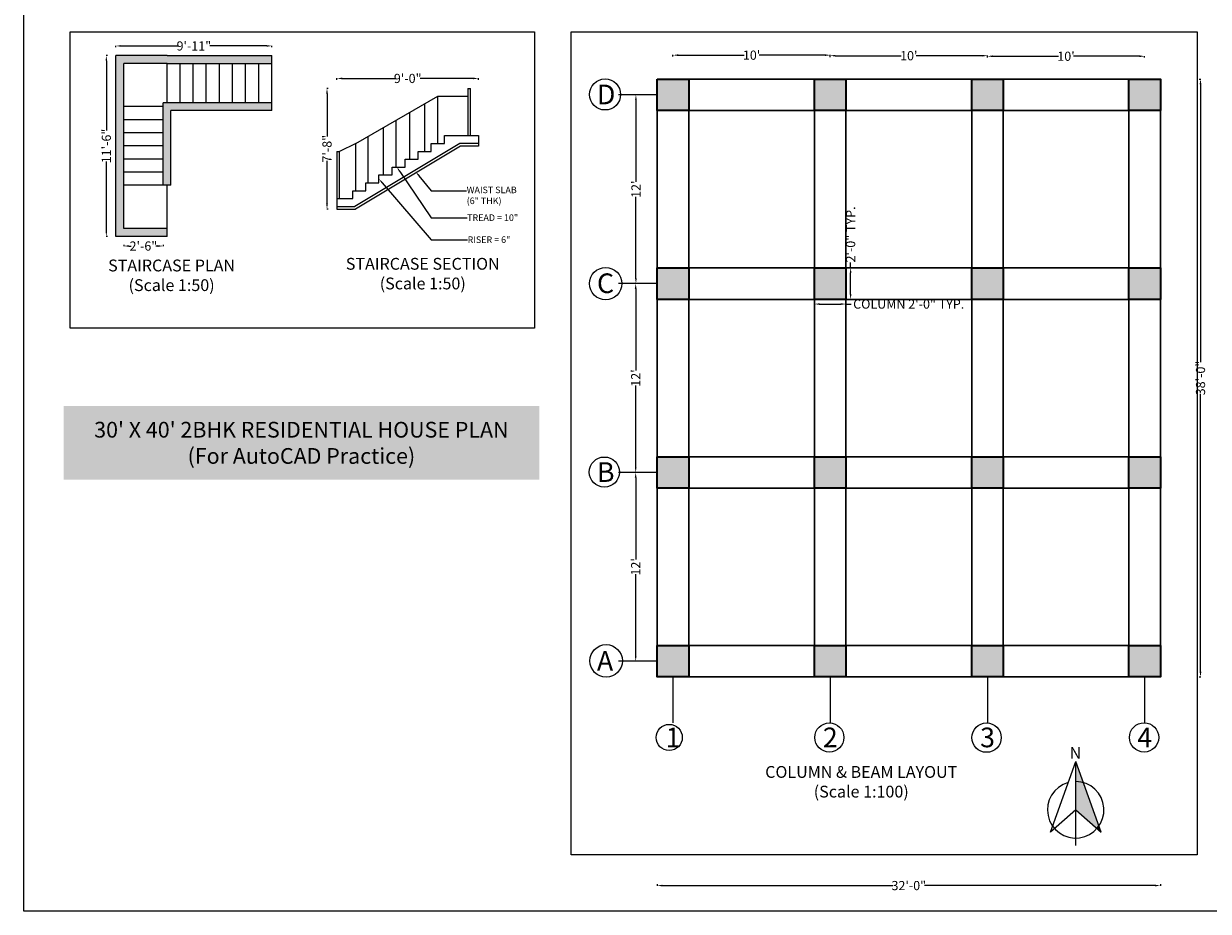
# Model space of a CAD drawing. Units: inches. Extents: x -80 to 1461, y -1239 to 153.
# Tile 1 of 6: x -80 to 824, y -1239 to -562. Entities that reach past the tile are written whole.
import ezdxf
from ezdxf import colors
from ezdxf.entities.mleader import LeaderData, LeaderLine
from ezdxf.math import Vec2, Vec3

# ---------------------------------------------------------------- set-up
doc = ezdxf.new("R2010")
doc.units = ezdxf.units.IN
doc.header["$MEASUREMENT"] = 0
for name, color, linetype, lineweight in [('A-ANNO-DIMS', 2, 'Continuous', 18), ('A-ANNO-SYMB', 3, 'Continuous', 18), ('A-ANNO-TEXT', 7, 'Continuous', 18), ('A-ANNO-TTLB', 7, 'Continuous', 25), ('A-DETL', 7, 'Continuous', 25), ('A-DETL-PATT', 8, 'Continuous', 13), ('A-FLOR-STRS', 7, 'Continuous', 20), ('A-GRID', 5, 'Continuous', 18), ('S-BEAM', 3, 'Continuous', 30), ('S-COLS', 7, 'Continuous', 35), ('S-COLS-PATT', 8, 'Continuous', 13)]:
    doc.layers.add(name, color=color, linetype=linetype, lineweight=lineweight)
doc.styles.get("Standard").update_dxf_attribs({"font": 'arial.ttf'})
doc.dimstyles.get("Standard").update_dxf_attribs({"dimtxt": 7, "dimasz": 4, "dimexe": 0.18, "dimexo": 0.0625, "dimgap": 0.09, "dimtad": 0, "dimdec": 0, "dimzin": 0, "dimdsep": 46, "dimlunit": 3, "dimtxsty": 'Standard', "dimcen": 0.09, "dimadec": 0, "dimazin": 0, "dimtfac": 1, "dimtdec": 0, "dimtofl": 0, "dimtmove": 0, "dimatfit": 3, "dimfxl": 1, "dimfxlon": 1, "dimtolj": 1, "dimtzin": 0, "dimarcsym": 0})

# ---------------------------------------------------------------- blocks, each defined once
blk = doc.blocks.new('*D15')
at = {"layer": 'A-ANNO-DIMS', "color": 0, "lineweight": -2, "transparency": 16777216}
for p, q in [((415.7, -587.34), (415.7, -586.16)), ((419.7, -586.34), (470, -586.34)), ((531.7, -586.34), (481.4, -586.34)), ((535.7, -587.34), (535.7, -586.16))]:
    blk.add_line(p, q, dxfattribs=at)
at = {"layer": 'A-ANNO-DIMS', "color": 0, "transparency": 16777216}
for points in [[(419.7, -585.67), (419.7, -587), (415.7, -586.34)], [(531.7, -585.67), (531.7, -587), (535.7, -586.34)]]:
    blk.add_solid(points, dxfattribs=at)
at = {"layer": 'Defpoints', "color": 0, "transparency": 16777216}
for p in [(535.7, -586.34), (415.7, -604.56), (535.7, -604.56)]:
    blk.add_point(p, dxfattribs=at)
at = {"layer": 'A-ANNO-DIMS', "color": 0, "transparency": 16777216, "insert": (475.7, -586.34), "char_height": 7, "attachment_point": 5}
blk.add_mtext("\\A1;10'", dxfattribs=at)
blk = doc.blocks.new('*D16')
at = {"layer": 'A-ANNO-DIMS', "color": 0, "lineweight": -2, "transparency": 16777216}
for p, q in [((535.7, -587.75), (535.7, -586.57)), ((539.7, -586.75), (590, -586.75)), ((651.7, -586.75), (601.4, -586.75)), ((655.7, -587.75), (655.7, -586.57))]:
    blk.add_line(p, q, dxfattribs=at)
at = {"layer": 'A-ANNO-DIMS', "color": 0, "transparency": 16777216}
for points in [[(539.7, -586.08), (539.7, -587.41), (535.7, -586.75)], [(651.7, -586.08), (651.7, -587.41), (655.7, -586.75)]]:
    blk.add_solid(points, dxfattribs=at)
at = {"layer": 'Defpoints', "color": 0, "transparency": 16777216}
for p in [(655.7, -586.75), (535.7, -604.56), (655.7, -604.56)]:
    blk.add_point(p, dxfattribs=at)
at = {"layer": 'A-ANNO-DIMS', "color": 0, "transparency": 16777216, "insert": (595.7, -586.75), "char_height": 7, "attachment_point": 5}
blk.add_mtext("\\A1;10'", dxfattribs=at)
blk = doc.blocks.new('*D17')
at = {"layer": 'A-ANNO-DIMS', "color": 0, "lineweight": -2, "transparency": 16777216}
for p, q in [((655.7, -588.16), (655.7, -586.98)), ((659.7, -587.16), (710, -587.16)), ((771.7, -587.16), (721.4, -587.16)), ((775.7, -588.16), (775.7, -586.98))]:
    blk.add_line(p, q, dxfattribs=at)
at = {"layer": 'A-ANNO-DIMS', "color": 0, "transparency": 16777216}
for points in [[(659.7, -586.49), (659.7, -587.82), (655.7, -587.16)], [(771.7, -586.49), (771.7, -587.82), (775.7, -587.16)]]:
    blk.add_solid(points, dxfattribs=at)
at = {"layer": 'Defpoints', "color": 0, "transparency": 16777216}
for p in [(775.7, -587.16), (655.7, -604.56), (775.7, -604.56)]:
    blk.add_point(p, dxfattribs=at)
at = {"layer": 'A-ANNO-DIMS', "color": 0, "transparency": 16777216, "insert": (715.7, -587.16), "char_height": 7, "attachment_point": 5}
blk.add_mtext("\\A1;10'", dxfattribs=at)
blk = doc.blocks.new('*D18')
at = {"layer": 'A-ANNO-DIMS', "color": 0, "lineweight": -2, "transparency": 16777216}
for p, q in [((388.44, -616.56), (387.26, -616.56)), ((387.44, -620.56), (387.44, -682.86)), ((387.44, -756.56), (387.44, -694.26)), ((388.44, -760.56), (387.26, -760.56))]:
    blk.add_line(p, q, dxfattribs=at)
at = {"layer": 'A-ANNO-DIMS', "color": 0, "transparency": 16777216}
for points in [[(386.77, -620.56), (388.11, -620.56), (387.44, -616.56)], [(386.77, -756.56), (388.11, -756.56), (387.44, -760.56)]]:
    blk.add_solid(points, dxfattribs=at)
at = {"layer": 'Defpoints', "color": 0, "transparency": 16777216}
for p in [(403.7, -616.56), (387.44, -760.56), (403.7, -760.56)]:
    blk.add_point(p, dxfattribs=at)
at = {"layer": 'A-ANNO-DIMS', "color": 0, "transparency": 16777216, "insert": (387.44, -688.56), "char_height": 7, "attachment_point": 5, "rotation": 90}
blk.add_mtext("\\A1;12'", dxfattribs=at)
blk = doc.blocks.new('*D19')
at = {"layer": 'A-ANNO-DIMS', "color": 0, "lineweight": -2, "transparency": 16777216}
for p, q in [((388.26, -760.56), (387.08, -760.56)), ((387.26, -764.56), (387.26, -826.86)), ((387.26, -900.56), (387.26, -838.26)), ((388.26, -904.56), (387.08, -904.56))]:
    blk.add_line(p, q, dxfattribs=at)
at = {"layer": 'A-ANNO-DIMS', "color": 0, "transparency": 16777216}
for points in [[(386.59, -764.56), (387.93, -764.56), (387.26, -760.56)], [(386.59, -900.56), (387.93, -900.56), (387.26, -904.56)]]:
    blk.add_solid(points, dxfattribs=at)
at = {"layer": 'Defpoints', "color": 0, "transparency": 16777216}
for p in [(403.7, -760.56), (387.26, -904.56), (403.7, -904.56)]:
    blk.add_point(p, dxfattribs=at)
at = {"layer": 'A-ANNO-DIMS', "color": 0, "transparency": 16777216, "insert": (387.26, -832.56), "char_height": 7, "attachment_point": 5, "rotation": 90}
blk.add_mtext("\\A1;12'", dxfattribs=at)
blk = doc.blocks.new('*D20')
at = {"layer": 'A-ANNO-DIMS', "color": 0, "lineweight": -2, "transparency": 16777216}
for p, q in [((388.26, -904.56), (387.08, -904.56)), ((387.26, -908.56), (387.26, -970.86)), ((387.26, -1044.56), (387.26, -982.26)), ((388.26, -1048.56), (387.08, -1048.56))]:
    blk.add_line(p, q, dxfattribs=at)
at = {"layer": 'A-ANNO-DIMS', "color": 0, "transparency": 16777216}
for points in [[(386.59, -908.56), (387.93, -908.56), (387.26, -904.56)], [(386.59, -1044.56), (387.93, -1044.56), (387.26, -1048.56)]]:
    blk.add_solid(points, dxfattribs=at)
at = {"layer": 'Defpoints', "color": 0, "transparency": 16777216}
for p in [(403.7, -904.56), (387.26, -1048.56), (403.7, -1048.56)]:
    blk.add_point(p, dxfattribs=at)
at = {"layer": 'A-ANNO-DIMS', "color": 0, "transparency": 16777216, "insert": (387.26, -976.56), "char_height": 7, "attachment_point": 5, "rotation": 90}
blk.add_mtext("\\A1;12'", dxfattribs=at)
blk = doc.blocks.new('COLUMN-24X24')
blk.add_lwpolyline([(0, 24), (24, 24), (24, 0), (0, 0)], close=True)
blk = doc.blocks.new('*D34')
at = {"layer": 'A-ANNO-DIMS', "color": 0, "lineweight": -2, "transparency": 16777216}
for p, q in [((523.7, -775.16), (523.7, -776.34)), ((527.7, -776.16), (543.7, -776.16)), ((547.7, -775.16), (547.7, -776.34)), ((547.7, -776.16), (551.7, -776.16))]:
    blk.add_line(p, q, dxfattribs=at)
at = {"layer": 'A-ANNO-DIMS', "color": 0, "transparency": 16777216}
for points in [[(527.7, -775.5), (527.7, -776.83), (523.7, -776.16)], [(543.7, -775.5), (543.7, -776.83), (547.7, -776.16)]]:
    blk.add_solid(points, dxfattribs=at)
at = {"layer": 'Defpoints', "color": 0, "transparency": 16777216}
for p in [(523.7, -772.56), (547.7, -772.56), (547.7, -776.16)]:
    blk.add_point(p, dxfattribs=at)
at = {"layer": 'A-ANNO-DIMS', "color": 0, "transparency": 16777216, "insert": (595.63, -776.16), "char_height": 7, "attachment_point": 5}
blk.add_mtext('\\A1;COLUMN 2\'-0" TYP.', dxfattribs=at)
blk = doc.blocks.new('*D35')
at = {"layer": 'A-ANNO-DIMS', "color": 0, "lineweight": -2, "transparency": 16777216}
for p, q in [((550.3, -748.56), (551.48, -748.56)), ((551.3, -748.56), (551.3, -744.56)), ((551.3, -768.56), (551.3, -752.56)), ((550.3, -772.56), (551.48, -772.56))]:
    blk.add_line(p, q, dxfattribs=at)
at = {"layer": 'A-ANNO-DIMS', "color": 0, "transparency": 16777216}
for points in [[(550.63, -752.56), (551.97, -752.56), (551.3, -748.56)], [(550.63, -768.56), (551.97, -768.56), (551.3, -772.56)]]:
    blk.add_solid(points, dxfattribs=at)
at = {"layer": 'Defpoints', "color": 0, "transparency": 16777216}
for p in [(547.7, -748.56), (551.3, -748.56), (547.7, -772.56)]:
    blk.add_point(p, dxfattribs=at)
at = {"layer": 'A-ANNO-DIMS', "color": 0, "transparency": 16777216, "insert": (551.3, -723.08), "char_height": 7, "attachment_point": 5, "rotation": 90}
blk.add_mtext('\\A1;2\'-0" TYP.', dxfattribs=at)
blk = doc.blocks.new('*D65')
at = {"layer": 'A-ANNO-DIMS', "color": 0, "lineweight": -2, "transparency": 16777216}
for p, q in [((-9.44, -580.3), (-9.44, -579.12)), ((-5.44, -579.3), (37.94, -579.3)), ((105.56, -579.3), (62.17, -579.3)), ((109.56, -580.3), (109.56, -579.12))]:
    blk.add_line(p, q, dxfattribs=at)
at = {"layer": 'A-ANNO-DIMS', "color": 0, "transparency": 16777216}
for points in [[(-5.44, -578.64), (-5.44, -579.97), (-9.44, -579.3)], [(105.56, -578.64), (105.56, -579.97), (109.56, -579.3)]]:
    blk.add_solid(points, dxfattribs=at)
at = {"layer": 'Defpoints', "color": 0, "transparency": 16777216}
for p in [(-9.44, -586.6), (109.56, -579.3), (109.56, -586.6)]:
    blk.add_point(p, dxfattribs=at)
at = {"layer": 'A-ANNO-DIMS', "color": 0, "transparency": 16777216, "insert": (50.06, -579.3), "char_height": 7, "attachment_point": 5}
blk.add_mtext('\\A1;9\'-11"', dxfattribs=at)
blk = doc.blocks.new('*D66')
at = {"layer": 'A-ANNO-DIMS', "color": 0, "lineweight": -2, "transparency": 16777216}
for p, q in [((-15.74, -586.6), (-16.92, -586.6)), ((-16.74, -590.6), (-16.74, -643.82)), ((-16.74, -720.6), (-16.74, -667.39)), ((-15.74, -724.6), (-16.92, -724.6))]:
    blk.add_line(p, q, dxfattribs=at)
at = {"layer": 'A-ANNO-DIMS', "color": 0, "transparency": 16777216}
for points in [[(-17.41, -590.6), (-16.08, -590.6), (-16.74, -586.6)], [(-17.41, -720.6), (-16.08, -720.6), (-16.74, -724.6)]]:
    blk.add_solid(points, dxfattribs=at)
at = {"layer": 'Defpoints', "color": 0, "transparency": 16777216}
for p in [(-9.44, -586.6), (-16.74, -724.6), (-9.44, -724.6)]:
    blk.add_point(p, dxfattribs=at)
at = {"layer": 'A-ANNO-DIMS', "color": 0, "transparency": 16777216, "insert": (-16.74, -655.6), "char_height": 7, "attachment_point": 5, "rotation": 90}
blk.add_mtext('\\A1;11\'-6"', dxfattribs=at)
blk = doc.blocks.new('*D67')
at = {"layer": 'A-ANNO-DIMS', "color": 0, "lineweight": -2, "transparency": 16777216}
for p, q in [((-3.44, -730.9), (-3.44, -732.08)), ((0.56, -731.9), (2.1, -731.9)), ((22.56, -731.9), (21.01, -731.9)), ((26.56, -730.9), (26.56, -732.08))]:
    blk.add_line(p, q, dxfattribs=at)
at = {"layer": 'A-ANNO-DIMS', "color": 0, "transparency": 16777216}
for points in [[(0.56, -731.24), (0.56, -732.57), (-3.44, -731.9)], [(22.56, -731.24), (22.56, -732.57), (26.56, -731.9)]]:
    blk.add_solid(points, dxfattribs=at)
at = {"layer": 'Defpoints', "color": 0, "transparency": 16777216}
for p in [(-3.44, -685.6), (26.56, -685.6), (26.56, -731.9)]:
    blk.add_point(p, dxfattribs=at)
at = {"layer": 'A-ANNO-DIMS', "color": 0, "transparency": 16777216, "insert": (11.56, -731.9), "char_height": 7, "attachment_point": 5}
blk.add_mtext('\\A1;2\'-6"', dxfattribs=at)
blk = doc.blocks.new('*D68')
at = {"layer": 'A-ANNO-DIMS', "color": 0, "lineweight": -2, "transparency": 16777216}
for p, q in [((159.28, -605.09), (159.28, -603.91)), ((163.28, -604.09), (203.87, -604.09)), ((263.25, -604.09), (222.66, -604.09)), ((267.25, -605.09), (267.25, -603.91))]:
    blk.add_line(p, q, dxfattribs=at)
at = {"layer": 'A-ANNO-DIMS', "color": 0, "transparency": 16777216}
for points in [[(163.28, -603.42), (163.28, -604.75), (159.28, -604.09)], [(263.25, -603.42), (263.25, -604.75), (267.25, -604.09)]]:
    blk.add_solid(points, dxfattribs=at)
at = {"layer": 'Defpoints', "color": 0, "transparency": 16777216}
for p in [(267.25, -604.09), (267.25, -655.69), (159.28, -703.69)]:
    blk.add_point(p, dxfattribs=at)
at = {"layer": 'A-ANNO-DIMS', "color": 0, "transparency": 16777216, "insert": (213.26, -604.09), "char_height": 7, "attachment_point": 5}
blk.add_mtext('\\A1;9\'-0"', dxfattribs=at)
blk = doc.blocks.new('*D69')
at = {"layer": 'A-ANNO-DIMS', "color": 0, "lineweight": -2, "transparency": 16777216}
for p, q in [((152.68, -611.69), (151.5, -611.69)), ((151.68, -615.69), (151.68, -648.32)), ((151.68, -699.69), (151.68, -667.05)), ((152.68, -703.69), (151.5, -703.69))]:
    blk.add_line(p, q, dxfattribs=at)
at = {"layer": 'A-ANNO-DIMS', "color": 0, "transparency": 16777216}
for points in [[(151.01, -615.69), (152.34, -615.69), (151.68, -611.69)], [(151.01, -699.69), (152.34, -699.69), (151.68, -703.69)]]:
    blk.add_solid(points, dxfattribs=at)
at = {"layer": 'Defpoints', "color": 0, "transparency": 16777216}
for p in [(151.68, -611.69), (259.26, -611.69), (159.28, -703.69)]:
    blk.add_point(p, dxfattribs=at)
at = {"layer": 'A-ANNO-DIMS', "color": 0, "transparency": 16777216, "insert": (151.68, -657.69), "char_height": 7, "attachment_point": 5, "rotation": 90}
blk.add_mtext('\\A1;7\'-8"', dxfattribs=at)
blk = doc.blocks.new('*D70')
at = {"layer": 'A-ANNO-DIMS', "color": 0, "lineweight": -2, "transparency": 16777216}
for p, q in [((403.7, -1218.66), (403.7, -1219.84)), ((407.7, -1219.66), (583.59, -1219.66)), ((783.7, -1219.66), (607.81, -1219.66)), ((787.7, -1218.66), (787.7, -1219.84))]:
    blk.add_line(p, q, dxfattribs=at)
at = {"layer": 'A-ANNO-DIMS', "color": 0, "transparency": 16777216}
for points in [[(407.7, -1219), (407.7, -1220.33), (403.7, -1219.66)], [(783.7, -1219), (783.7, -1220.33), (787.7, -1219.66)]]:
    blk.add_solid(points, dxfattribs=at)
at = {"layer": 'Defpoints', "color": 0, "transparency": 16777216}
for p in [(403.7, -1060.56), (787.7, -1060.56), (787.7, -1219.66)]:
    blk.add_point(p, dxfattribs=at)
at = {"layer": 'A-ANNO-DIMS', "color": 0, "transparency": 16777216, "insert": (595.7, -1219.66), "char_height": 7, "attachment_point": 5}
blk.add_mtext('\\A1;32\'-0"', dxfattribs=at)
blk = doc.blocks.new('*D71')
at = {"layer": 'A-ANNO-DIMS', "color": 0, "lineweight": -2, "transparency": 16777216}
for p, q in [((817.33, -604.56), (818.51, -604.56)), ((818.33, -608.56), (818.33, -820.45)), ((818.33, -1056.56), (818.33, -844.67)), ((817.33, -1060.56), (818.51, -1060.56))]:
    blk.add_line(p, q, dxfattribs=at)
at = {"layer": 'A-ANNO-DIMS', "color": 0, "transparency": 16777216}
for points in [[(817.66, -608.56), (818.99, -608.56), (818.33, -604.56)], [(817.66, -1056.56), (818.99, -1056.56), (818.33, -1060.56)]]:
    blk.add_solid(points, dxfattribs=at)
at = {"layer": 'Defpoints', "color": 0, "transparency": 16777216}
for p in [(787.7, -604.56), (818.33, -604.56), (787.7, -1060.56)]:
    blk.add_point(p, dxfattribs=at)
at = {"layer": 'A-ANNO-DIMS', "color": 0, "transparency": 16777216, "insert": (818.33, -832.56), "char_height": 7, "attachment_point": 5, "rotation": 90}
blk.add_mtext('\\A1;38\'-0"', dxfattribs=at)

msp = doc.modelspace()

# ---------------------------------------------------------------- hatches: boundary and pattern name
at = {"layer": 'A-ANNO-SYMB'}
h = msp.add_hatch(color=256, dxfattribs=at)
h.dxf.hatch_style = 1
h.paths.add_polyline_path([(728.85, -1141.11, 0.067956), (723.07, -1140.32), (723.07, -1161.88), (739.23, -1176.15, 0.028033), (740.73, -1174.26)])
h.paths.add_polyline_path([(723.07, -1124.97), (723.07, -1140.32, -0.067956), (728.85, -1141.11)])
h = msp.add_hatch(color=256, dxfattribs=at)
h.dxf.hatch_style = 1
h.paths.add_polyline_path([(740.73, -1174.26, -0.028033), (739.23, -1176.15), (742.42, -1178.96)])
at = {"layer": 'A-DETL-PATT'}
h = msp.add_hatch(dxfattribs=at)
h.set_pattern_fill('AR-CONC', color=256, scale=0.2)
h.set_pattern_definition([(50, (-362.7912, 212.4004), (1.4345204, -0.1255043), [0.15, -1.65]), (355, (-362.7912, 212.4004), (-0.2775027, 1.5043843), [0.12, -1.32]), (100.45144, (-362.6716, 212.39), (1.1570177, 1.37888), [0.1274804, -1.4022842]), (46.1842, (-362.7912, 212.8004), (2.1344827, -0.3310386), [0.225, -2.475]), (96.63564, (-362.6133, 212.7728), (1.869324, 1.948237), [0.1912207, -2.1034275]), (351.18416, (-362.7912, 212.8004), (1.869324, 1.948237), [0.18, -1.98]), (21, (-362.5912, 212.7004), (1.1938141, -0.8052378), [0.15, -1.65]), (326, (-362.5912, 212.7004), (0.4866307, 1.4503), [0.12, -1.32]), (71.45144, (-362.4917, 212.6333), (1.6804448, 0.6450623), [0.1274804, -1.4022842]), (37.5, (-362.79116, 212.4004), (0.0243197, 0.6657877), [0, -1.304, 0, -1.34, 0, -1.325]), (7.5, (-362.79116, 212.4004), (0.52613907, 0.7888234), [0, -0.764, 0, -1.274, 0, -0.505]), (327.5, (-363.23716, 212.4004), (1.06764487, -0.04510974), [0, -0.5, 0, -1.56, 0, -2.07]), (317.5, (-363.4372, 212.4004), (1.1663723, 0.20021), [0, -0.65, 0, -1.036, 0, -1.47])])
h.paths.add_polyline_path([(29.56, -592.6), (109.56, -592.6), (109.56, -586.6), (29.56, -586.6), (-9.44, -586.6), (-9.44, -685.6), (-9.44, -724.6), (29.56, -724.6), (29.56, -718.6), (-3.44, -718.6), (-3.44, -685.6), (-3.44, -592.6)])
h.paths.add_polyline_path([(109.56, -628.6), (109.56, -622.6), (26.56, -622.6), (26.56, -685.6), (32.56, -685.6), (32.56, -628.6)], flags=17)
at = {"layer": 'S-COLS-PATT'}
h = msp.add_hatch(dxfattribs=at)
h.set_pattern_fill('AR-CONC', color=256)
h.set_pattern_definition([(50, (-29.1613, 49.472), (7.172602, -0.627521), [0.75, -8.25]), (355, (-29.161, 49.472), (-1.387513, 7.52192), [0.6, -6.6]), (100.45144, (-28.5636, 49.4195), (5.78509, 6.8944), [0.637402, -7.01142]), (46.1842, (-29.161, 51.472), (10.672413, -1.65519), [1.125, -12.375]), (96.6356, (-28.272, 51.334), (9.34662, 9.741186), [0.9561, -10.51714]), (351.1842, (-29.161, 51.472), (9.34662, 9.74119), [0.9, -9.9]), (21, (-28.1613, 50.972), (5.96907, -4.02619), [0.75, -8.25]), (326, (-28.161, 50.972), (2.433153, 7.2515), [0.6, -6.6]), (71.45144, (-27.664, 50.636), (8.402224, 3.22531), [0.6374, -7.01142]), (37.5, (-29.1613, 49.4718), (0.1215986, 3.3289385), [0, -6.52, 0, -6.7, 0, -6.625]), (7.5, (-29.1613, 49.4718), (2.630695, 3.944117), [0, -3.82, 0, -6.37, 0, -2.525]), (327.5, (-31.3913, 49.4718), (5.3382244, -0.2255487), [0, -2.5, 0, -7.8, 0, -10.35]), (317.5, (-32.3913, 49.472), (5.831862, 1.00105), [0, -3.25, 0, -5.18, 0, -7.35])])
h.paths.add_polyline_path([(403.7, -604.56), (403.7, -628.56), (427.7, -628.56), (427.7, -604.56)])
h.paths.add_polyline_path([(523.7, -628.56), (547.7, -628.56), (547.7, -604.56), (523.7, -604.56)])
h.paths.add_polyline_path([(667.7, -604.56), (643.7, -604.56), (643.7, -628.56), (667.7, -628.56)])
h.paths.add_polyline_path([(763.7, -604.56), (763.7, -628.56), (787.7, -628.56), (787.7, -604.56)])
h.paths.add_polyline_path([(763.7, -748.56), (763.7, -772.56), (787.7, -772.56), (787.7, -748.56)])
h.paths.add_polyline_path([(667.7, -748.56), (643.7, -748.56), (643.7, -772.56), (667.7, -772.56)])
h.paths.add_polyline_path([(547.7, -748.56), (523.7, -748.56), (523.7, -772.56), (547.7, -772.56)])
h.paths.add_polyline_path([(427.7, -748.56), (403.7, -748.56), (403.7, -772.56), (427.7, -772.56)])
h.paths.add_polyline_path([(427.7, -892.56), (403.7, -892.56), (403.7, -916.56), (427.7, -916.56)])
h.paths.add_polyline_path([(523.7, -916.56), (547.7, -916.56), (547.7, -892.56), (523.7, -892.56)])
h.paths.add_polyline_path([(667.7, -916.56), (667.7, -892.56), (643.7, -892.56), (643.7, -916.56)])
h.paths.add_polyline_path([(787.7, -892.56), (763.7, -892.56), (763.7, -916.56), (787.7, -916.56)])
h.paths.add_polyline_path([(763.7, -1036.56), (763.7, -1060.56), (787.7, -1060.56), (787.7, -1036.56)])
h.paths.add_polyline_path([(643.7, -1036.56), (643.7, -1060.56), (667.7, -1060.56), (667.7, -1036.56)])
h.paths.add_polyline_path([(523.7, -1036.56), (523.7, -1060.56), (547.7, -1060.56), (547.7, -1036.56)])
h.paths.add_polyline_path([(427.7, -1036.56), (403.7, -1036.56), (403.7, -1060.56), (427.7, -1060.56)])

# ---------------------------------------------------------------- linework, layer by layer
at = {"layer": 'A-ANNO-SYMB'}
for p, q in [((703.73, -1178.96), (723.07, -1124.97)), ((742.42, -1178.96), (723.07, -1124.97)), ((723.07, -1189.04), (723.07, -1124.97)), ((723.07, -1161.88), (703.73, -1178.96)), ((723.07, -1161.88), (742.42, -1178.96))]:
    msp.add_line(p, q, dxfattribs=at)
msp.add_arc((723.07, -1161.88), 21.56, 105.55035, 90, dxfattribs=at)
at = {"layer": 'A-ANNO-TTLB'}
for points in [[(-79.81, 141.36), (1461.09, 141.36), (1461.09, -1239.28), (-79.81, -1239.28)], [(-44.36, -568.66), (310.08, -568.66), (310.08, -794.55), (-44.36, -794.55)], [(337.97, -568.66), (815.84, -568.66), (815.84, -1196.23), (337.97, -1196.23)]]:
    msp.add_lwpolyline(points, close=True, dxfattribs=at)
at = {"layer": 'A-DETL'}
for p, q in [((259.26, -611.69), (259.26, -647.69)), ((259.26, -611.69), (261.26, -611.69)), ((261.26, -647.69), (261.26, -611.69)), ((173.59, -653.69), (236.28, -617.69)), ((226.28, -659.69), (226.28, -623.43)), ((236.28, -653.69), (236.28, -617.69)), ((236.28, -617.69), (259.26, -617.69)), ((214.81, -665.69), (214.81, -630.01)), ((194.84, -677.69), (194.84, -641.48)), ((204.35, -671.69), (204.35, -636.02)), ((183.21, -683.69), (183.21, -648.16)), ((241.28, -653.69), (241.28, -647.69)), ((241.28, -647.69), (251.28, -647.69)), ((251.28, -647.69), (267.25, -647.69)), ((259.26, -647.69), (261.26, -647.69)), ((267.25, -647.69), (267.25, -653.69)), ((159.28, -659.69), (159.28, -695.69)), ((159.28, -659.69), (161.28, -659.69)), ((173.59, -653.69), (161.28, -659.69)), ((161.28, -695.69), (161.28, -659.69)), ((173.59, -689.69), (173.59, -653.69)), ((221.28, -665.69), (221.28, -659.69)), ((221.28, -659.69), (231.28, -659.69)), ((231.28, -659.69), (231.28, -653.69)), ((231.28, -653.69), (241.28, -653.69)), ((267.25, -653.69), (252.94, -653.69)), ((267.25, -655.69), (253.49, -655.69)), ((267.25, -653.69), (267.25, -655.69)), ((211.28, -671.69), (211.28, -665.69)), ((211.28, -665.69), (221.28, -665.69)), ((191.28, -683.69), (191.28, -677.69)), ((191.28, -677.69), (201.28, -677.69)), ((201.28, -677.69), (201.28, -671.69)), ((201.28, -671.69), (211.28, -671.69)), ((181.28, -689.69), (181.28, -683.69)), ((181.28, -683.69), (191.28, -683.69)), ((159.28, -695.69), (171.28, -695.69)), ((159.28, -695.69), (159.28, -701.69)), ((159.28, -695.69), (161.28, -695.69)), ((171.28, -695.69), (171.28, -689.69)), ((171.28, -689.69), (181.28, -689.69)), ((159.28, -701.69), (172.94, -701.69)), ((159.28, -701.69), (159.28, -703.69)), ((159.28, -703.69), (173.49, -703.69))]:
    msp.add_line(p, q, dxfattribs=at)
for points in [[(252.94, -653.69), (172.94, -701.69)], [(253.49, -655.69), (173.49, -703.69)]]:
    msp.add_lwpolyline(points, dxfattribs=at)
at = {"layer": 'A-FLOR-STRS'}
for p, q in [((-9.44, -685.6), (-9.44, -586.6)), ((29.56, -586.6), (-9.44, -586.6)), ((29.56, -586.6), (109.56, -586.6)), ((109.56, -628.6), (109.56, -586.6)), ((-3.44, -685.6), (-3.44, -592.6)), ((29.56, -592.6), (-3.44, -592.6)), ((29.56, -622.6), (29.56, -592.6)), ((29.56, -592.6), (109.56, -592.6)), ((39.56, -622.6), (39.56, -592.6)), ((49.56, -622.6), (49.56, -592.6)), ((59.56, -622.6), (59.56, -592.6)), ((69.56, -622.6), (69.56, -592.6)), ((79.56, -622.6), (79.56, -592.6)), ((89.56, -622.6), (89.56, -592.6)), ((99.56, -622.6), (99.56, -592.6)), ((26.56, -685.6), (26.56, -622.6)), ((109.56, -622.6), (26.56, -622.6)), ((26.56, -625.6), (-3.44, -625.6)), ((32.56, -685.6), (32.56, -628.6)), ((109.56, -628.6), (32.56, -628.6)), ((26.56, -635.6), (-3.44, -635.6)), ((26.56, -645.6), (-3.44, -645.6)), ((26.56, -655.6), (-3.44, -655.6)), ((26.56, -665.6), (-3.44, -665.6)), ((26.56, -675.6), (-3.44, -675.6)), ((-9.44, -724.6), (-9.44, -685.6)), ((-3.44, -718.6), (-3.44, -685.6)), ((32.56, -685.6), (-3.44, -685.6)), ((29.56, -724.6), (29.56, -685.6)), ((29.56, -718.6), (-3.44, -718.6)), ((29.56, -724.6), (-9.44, -724.6))]:
    msp.add_line(p, q, dxfattribs=at)
at = {"layer": 'A-GRID'}
for p, q in [((403.7, -616.56), (374.23, -616.56)), ((403.7, -760.56), (374.23, -760.56)), ((403.7, -904.56), (374.23, -904.56)), ((403.7, -1048.56), (374.23, -1048.56)), ((415.7, -1060.56), (415.7, -1095.46)), ((535.7, -1060.56), (535.7, -1095.46)), ((655.7, -1060.56), (655.7, -1095.46)), ((775.7, -1060.56), (775.7, -1095.46))]:
    msp.add_line(p, q, dxfattribs=at)
for centre, radius in [((363.89, -616.31), 11.84), ((364.32, -760.57), 12.32), ((363.36, -904.31), 11.5), ((364.7, -1048.31), 12.38), ((412.87, -1106.71), 9.99), ((535.07, -1106.71), 11.11), ((655.02, -1106.84), 11.18), ((775.29, -1106.68), 11.21)]:
    msp.add_circle(centre, radius, dxfattribs=at)
at = {"layer": 'S-BEAM'}
for p, q in [((403.7, -604.56), (787.7, -604.56)), ((403.7, -604.56), (403.7, -1048.56)), ((415.7, -604.56), (535.7, -604.56)), ((427.7, -604.56), (427.7, -1048.56)), ((523.7, -604.56), (523.7, -1048.56)), ((547.7, -604.56), (547.7, -1048.56)), ((643.7, -604.56), (643.7, -1048.56)), ((667.7, -604.56), (667.7, -1048.56)), ((763.7, -604.56), (763.7, -1048.56)), ((787.7, -604.56), (787.7, -1048.56)), ((403.7, -628.56), (787.7, -628.56)), ((403.7, -748.56), (787.7, -748.56)), ((403.7, -772.56), (787.7, -772.56)), ((403.7, -892.56), (787.7, -892.56)), ((403.7, -916.56), (787.7, -916.56)), ((403.7, -1036.56), (787.7, -1036.56)), ((403.7, -1060.56), (787.7, -1060.56))]:
    msp.add_line(p, q, dxfattribs=at)

# ---------------------------------------------------------------- block references
at = {"layer": 'S-COLS'}
for p in [(403.7, -628.56), (523.7, -628.56), (643.7, -628.56), (763.7, -628.56), (403.7, -772.56), (523.7, -772.56), (643.7, -772.56), (763.7, -772.56), (403.7, -916.56), (523.7, -916.56), (643.7, -916.56), (763.7, -916.56), (403.7, -1060.56), (523.7, -1060.56), (643.7, -1060.56), (763.7, -1060.56)]:
    msp.add_blockref('COLUMN-24X24', p, dxfattribs=at)

# ---------------------------------------------------------------- texts
at = {"layer": 'A-ANNO-SYMB', "insert": (713.41, -1113.99), "char_height": 9, "attachment_point": 1}
msp.add_mtext_dynamic_manual_height_columns('\\pxqc;{\\fArial|b1|i0|c0|p34;N}', width=18.9576, gutter_width=1, heights=[0], dxfattribs=at)
at = {"layer": 'A-ANNO-TEXT', "char_height": 9, "attachment_point": 1}
for s, width, insert in [('\\pxqc;STAIRCASE SECTION\\P(Scale 1:50)', 144.0716, (152.72, -740.96)), ('\\pxqc;STAIRCASE PLAN\\P(Scale 1:50)', 115.3092, (-24.58, -742.24)), ('\\pxqc;COLUMN & BEAM LAYOUT\\P(Scale 1:100)', 167.6365, (475.59, -1128.5))]:
    msp.add_mtext_dynamic_manual_height_columns(s, width=width, gutter_width=1, heights=[0], dxfattribs=dict(at, insert=insert))
at = {"layer": 'A-ANNO-TEXT', "insert": (-37.39, -866), "char_height": 12, "width": 339.0131, "attachment_point": 1, "bg_fill": 1, "box_fill_scale": 2, "bg_fill_color": 5, "bg_fill_transparency": 0}
msp.add_mtext("\\pxqc;30' X 40' 2BHK RESIDENTIAL HOUSE PLAN\\P(For AutoCAD Practice)", dxfattribs=at)
at = {"layer": 'A-GRID', "char_height": 15, "attachment_point": 1}
for s, insert in [('D', (357.69, -608.81)), ('C', (357.69, -752.81)), ('B', (357.69, -896.81)), ('A', (357.69, -1040.81)), ('1', (410.11, -1099.18)), ('2', (530.11, -1099.18)), ('3', (650.11, -1099.18)), ('4', (770.11, -1099.18))]:
    msp.add_mtext_dynamic_manual_height_columns(s, width=4.7941, gutter_width=1, heights=[0], dxfattribs=dict(at, insert=insert))

# ---------------------------------------------------------------- dimensions: what is measured, and where the dimension line sits
at = {"layer": 'A-ANNO-DIMS'}
for base, p1, p2, override, picture, middle in [((109.56, -579.3), (-9.44, -586.6), (109.56, -586.6), {"dimdec": 1, "dimlfac": 1, "dimrnd": 0, "dimzin": 1, "dimdsep": 46, "dimlunit": 4, "dimfrac": 2}, '*D65', (50.06, -579.3)), ((535.7, -586.34), (415.7, -604.56), (535.7, -604.56), {"dimclrd": 0, "dimclre": 0, "dimclrt": 0}, '*D15', (475.7, -586.34)), ((655.7, -586.75), (535.7, -604.56), (655.7, -604.56), {"dimclrd": 0, "dimclre": 0, "dimclrt": 0}, '*D16', (595.7, -586.75)), ((775.7, -587.16), (655.7, -604.56), (775.7, -604.56), {"dimclrd": 0, "dimclre": 0, "dimclrt": 0}, '*D17', (715.7, -587.16)), ((267.25, -604.09), (159.28, -703.69), (267.25, -655.69), {"dimdec": 1, "dimlfac": 1, "dimrnd": 0, "dimzin": 1, "dimdsep": 46, "dimlunit": 4, "dimfrac": 2}, '*D68', (213.26, -604.09)), ((26.56, -731.9), (-3.44, -685.6), (26.56, -685.6), {"dimdec": 1, "dimlfac": 1, "dimrnd": 0, "dimzin": 1, "dimdsep": 46, "dimlunit": 4, "dimfrac": 2}, '*D67', (11.56, -731.9)), ((787.7, -1219.66), (403.7, -1060.56), (787.7, -1060.56), {"dimdec": 1, "dimlfac": 1, "dimrnd": 0, "dimzin": 1, "dimdsep": 46, "dimlunit": 4, "dimfrac": 2}, '*D70', (595.7, -1219.66))]:
    dim = msp.add_linear_dim(base=base, p1=p1, p2=p2, dimstyle='Standard', override=override, dxfattribs=at)
    dim.commit()
    dim.dimension.update_dxf_attribs({"geometry": picture, "text_midpoint": middle})
for base, p1, p2, override, picture, middle in [((-16.74, -724.6), (-9.44, -586.6), (-9.44, -724.6), {"dimdec": 1, "dimlfac": 1, "dimrnd": 0, "dimzin": 1, "dimdsep": 46, "dimlunit": 4, "dimfrac": 2}, '*D66', (-16.74, -655.6)), ((818.33, -604.56), (787.7, -1060.56), (787.7, -604.56), {"dimdec": 1, "dimlfac": 1, "dimrnd": 0, "dimzin": 1, "dimdsep": 46, "dimlunit": 4, "dimfrac": 2}, '*D71', (818.33, -832.56)), ((151.68, -611.69), (159.28, -703.69), (259.26, -611.69), {"dimdec": 1, "dimlfac": 1, "dimrnd": 0, "dimzin": 1, "dimdsep": 46, "dimlunit": 4, "dimfrac": 2}, '*D69', (151.68, -657.69)), ((387.44, -760.56), (403.7, -616.56), (403.7, -760.56), {"dimclrd": 0, "dimclre": 0, "dimclrt": 0}, '*D18', (387.44, -688.56)), ((387.26, -904.56), (403.7, -760.56), (403.7, -904.56), {"dimclrd": 0, "dimclre": 0, "dimclrt": 0}, '*D19', (387.26, -832.56)), ((387.26, -1048.56), (403.7, -904.56), (403.7, -1048.56), {"dimclrd": 0, "dimclre": 0, "dimclrt": 0}, '*D20', (387.26, -976.56))]:
    dim = msp.add_linear_dim(base=base, p1=p1, p2=p2, angle=90, dimstyle='Standard', override=override, dxfattribs=at)
    dim.commit()
    dim.dimension.update_dxf_attribs({"geometry": picture, "text_midpoint": middle})
dim = msp.add_linear_dim(base=(551.3, -748.56), p1=(547.7, -772.56), p2=(547.7, -748.56), angle=90, text='<> TYP.', dimstyle='Standard', override={"dimdec": 1, "dimlfac": 1, "dimrnd": 0, "dimzin": 1, "dimdsep": 46, "dimlunit": 4, "dimfrac": 2}, dxfattribs=at)
dim.commit()
dim.dimension.update_dxf_attribs({"geometry": '*D35', "text_midpoint": (551.3, -723.08)})
dim = msp.add_linear_dim(base=(547.7, -776.16), p1=(523.7, -772.56), p2=(547.7, -772.56), text='COLUMN <> TYP.', dimstyle='Standard', override={"dimdec": 1, "dimlfac": 1, "dimrnd": 0, "dimzin": 1, "dimdsep": 46, "dimlunit": 4, "dimfrac": 2}, dxfattribs=at)
dim.commit()
dim.dimension.update_dxf_attribs({"geometry": '*D34', "text_midpoint": (595.63, -776.16)})

# ---------------------------------------------------------------- leaders
at = {"layer": 'A-ANNO-TEXT'}
ml = msp.add_multileader_mtext('Standard', dxfattribs=at)
ml.set_content('TREAD = 10"', color=256)
ml.set_leader_properties()
ml.build(insert=Vec2(0, 0))
ml.multileader.update_dxf_attribs({"dogleg_length": 0.36})
ctx = ml.context
ctx.base_point, ctx.char_height, ctx.landing_gap_size, ctx.plane_origin = Vec3(258.53, -710.29), 5, 0.09, Vec3(204.98, -671.69)
notes = []
notes.append((ctx, [(0, (1, 1, 0), (258.17, -710.29), (1, 0), 0.36, [(0, [(204.98, -671.69), (231.24, -710.29)], 0, [])])]))
ctx.mtext.insert, ctx.mtext.flow_direction = Vec3(258.62, -707.75), 5
ml = msp.add_multileader_mtext('Standard', dxfattribs=at)
ml.set_content('WAIST SLAB\\P(6" THK)', color=256)
ml.set_leader_properties()
ml.build(insert=Vec2(0, 0))
ml.multileader.update_dxf_attribs({"dogleg_length": 0.36})
ctx = ml.context
ctx.base_point, ctx.char_height, ctx.landing_gap_size, ctx.plane_origin = Vec3(258.17, -689.83), 5, 0.09, Vec3(219.33, -675.15)
notes.append((ctx, [(0, (1, 1, 0), (257.81, -689.83), (1, 0), 0.36, [(0, [(219.33, -675.15), (231.24, -689.83)], 0, [])])]))
ctx.mtext.insert, ctx.mtext.flow_direction = Vec3(258.26, -686.59), 5
ml = msp.add_multileader_mtext('Standard', dxfattribs=at)
ml.set_content('RISER = 6"', color=256)
ml.set_leader_properties()
ml.build(insert=Vec2(0, 0))
ml.multileader.update_dxf_attribs({"dogleg_length": 0.36})
ctx = ml.context
ctx.base_point, ctx.char_height, ctx.landing_gap_size, ctx.plane_origin = Vec3(258.89, -727.12), 5, 0.09, Vec3(191.28, -680.69)
notes.append((ctx, [(0, (1, 1, 0), (258.53, -727.12), (1, 0), 0.36, [(0, [(191.28, -680.69), (231.24, -727.12)], 0, [])])]))
ctx.mtext.insert, ctx.mtext.flow_direction = Vec3(258.98, -724.58), 5
for ctx, leaders in notes:
    for number, flags, end, landing, length, lines in leaders:
        leader = LeaderData()
        leader.index, (leader.has_last_leader_line, leader.has_dogleg_vector, leader.attachment_direction) = number, flags
        leader.last_leader_point, leader.dogleg_vector, leader.dogleg_length = Vec3(end), Vec3(landing), length
        for number, points, colour, breaks in lines:
            line = LeaderLine()
            line.index, line.vertices, line.color, line.breaks = number, Vec3.list(points), colors.encode_raw_color(colour), breaks
            leader.lines.append(line)
        ctx.leaders.append(leader)

doc.saveas('drawing.dxf')
